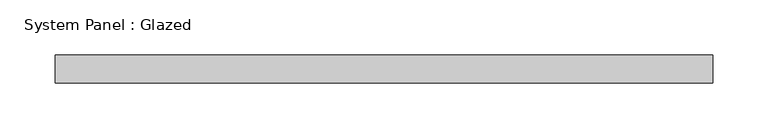
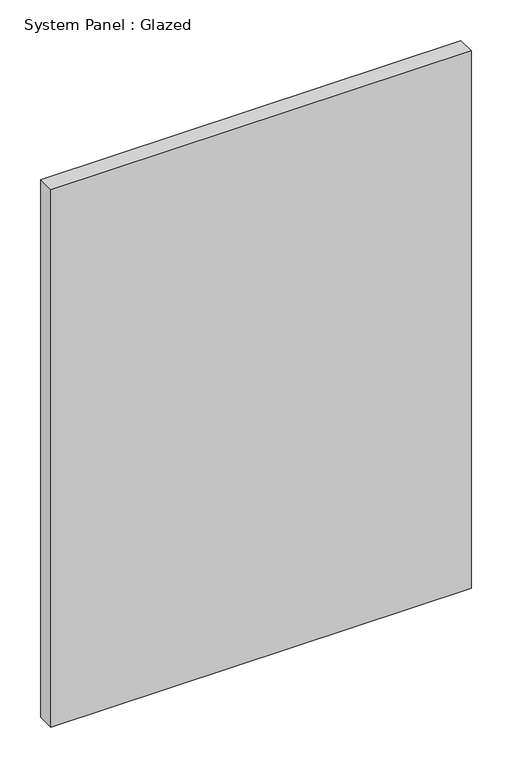
"""IFC4 building model written with IfcOpenShell, lengths in millimetres: plate geometry, System Panel : Glazed."""

from ifc_helpers import new_model, si_unit, origin, origin_with_axes, place, context, project, spatial, polyline, outline, extrude, source, transform, mapped, element, save


def system_panel_glazed_0523aacf(model_context):
    return source(origin(), model_context, "Body", "SweptSolid", [
        extrude(outline(polyline([(298.45, 19.05), (-298.45, 19.05), (-298.45, 44.45), (298.45, 44.45), (298.45, 19.05)])), origin_with_axes(), (0.0, 0.0, 1.0), 807.2801773),
    ])


if __name__ == "__main__":
    model = new_model("IFC4")
    model_context = context("Model", 3, world=origin())
    ifc_project = project(units=[si_unit("LENGTHUNIT", "METRE", prefix="MILLI")], contexts=[model_context])
    site = spatial("IfcSite", under=ifc_project)
    building = spatial("IfcBuilding", under=site)
    placement = place(None, origin())
    system_panel_glazed_shape = system_panel_glazed_0523aacf(model_context)
    element("IfcPlate", 1, ObjectType="System Panel : Glazed", at=placement, inside=building, context=model_context, shape_type="MappedRepresentation", body=[
        mapped(system_panel_glazed_shape, transform((0.0, 0.0, 0.0), x_axis=(1.0, 0.0, 0.0), y_axis=(0.0, 1.0, 0.0), z_axis=(0.0, 0.0, 1.0))),
    ])
    save(model, "model.ifc")

# Revit data of these elements
# Type "System Panel : Glazed"
#   Construction Type Id = "GSP4R"
#   Analytic Construction = "1/8 in Pilkington single glazing"
#   Visual Light Transmittance = 0.9
#   Solar Heat Gain Coefficient = 0.86
#   Heat Transfer Coefficient (U) = 1.18115 BTU/(h·ft²·°F)
#   Define Thermal Properties by = 1
# Element 1 (IfcPlate, "System Panel : Glazed")
#   Materials on its faces: "Glass"
# Materials
#   "Glass": class "Glass", colour RGB 0 128 192, transparency 0.75, Description = "Soda Lime Glass", Cost = 0
